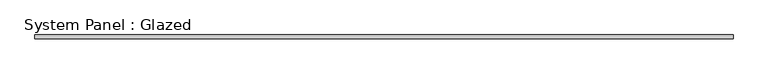
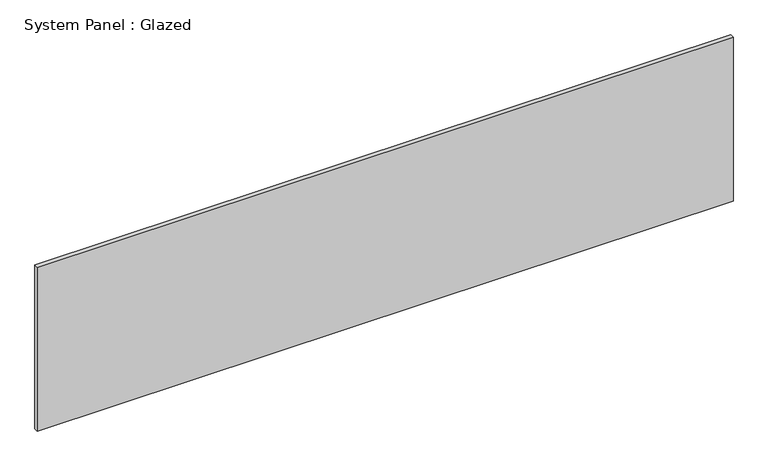
"""IFC4 building model written with IfcOpenShell, lengths in millimetres: plate geometry, System Panel : Glazed."""

from ifc_helpers import new_model, si_unit, origin, origin_with_axes, place, context, project, spatial, polyline, outline, extrude, source, transform, mapped, element, save


def system_panel_glazed_0c1985eb(model_context):
    return source(origin(), model_context, "Body", "SweptSolid", [
        extrude(outline(polyline([(2319.4141213, 19.05), (-2319.4141213, 19.05), (-2319.4141213, 44.45), (2319.4141213, 44.45), (2319.4141213, 19.05)])), origin_with_axes(), (0.0, 0.0, 1.0), 1155.7),
    ])


if __name__ == "__main__":
    model = new_model("IFC4")
    model_context = context("Model", 3, world=origin())
    ifc_project = project(units=[si_unit("LENGTHUNIT", "METRE", prefix="MILLI")], contexts=[model_context])
    site = spatial("IfcSite", under=ifc_project)
    building = spatial("IfcBuilding", under=site)
    placement = place(None, origin())
    system_panel_glazed_shape = system_panel_glazed_0c1985eb(model_context)
    element("IfcPlate", 1, ObjectType="System Panel : Glazed", at=placement, inside=building, context=model_context, shape_type="MappedRepresentation", body=[
        mapped(system_panel_glazed_shape, transform((0.0, 0.0, 0.0), x_axis=(1.0, 0.0, 0.0), y_axis=(0.0, 1.0, 0.0), z_axis=(0.0, 0.0, 1.0))),
    ])
    save(model, "model.ifc")

# Revit data of these elements
# Type "System Panel : Glazed"
#   Construction Type Id = "GSP4R"
#   Analytic Construction = "1/8 in Pilkington single glazing"
#   Visual Light Transmittance = 0.9
#   Solar Heat Gain Coefficient = 0.86
#   Heat Transfer Coefficient (U) = 1.18115 BTU/(h·ft²·°F)
# Element 1 (IfcPlate, "System Panel : Glazed")
#   Materials on its faces: "Glass"
# Materials
#   "Glass": class "Glass", colour RGB 0 128 192, transparency 0.75, Description = "Soda Lime Glass", Cost = 0
